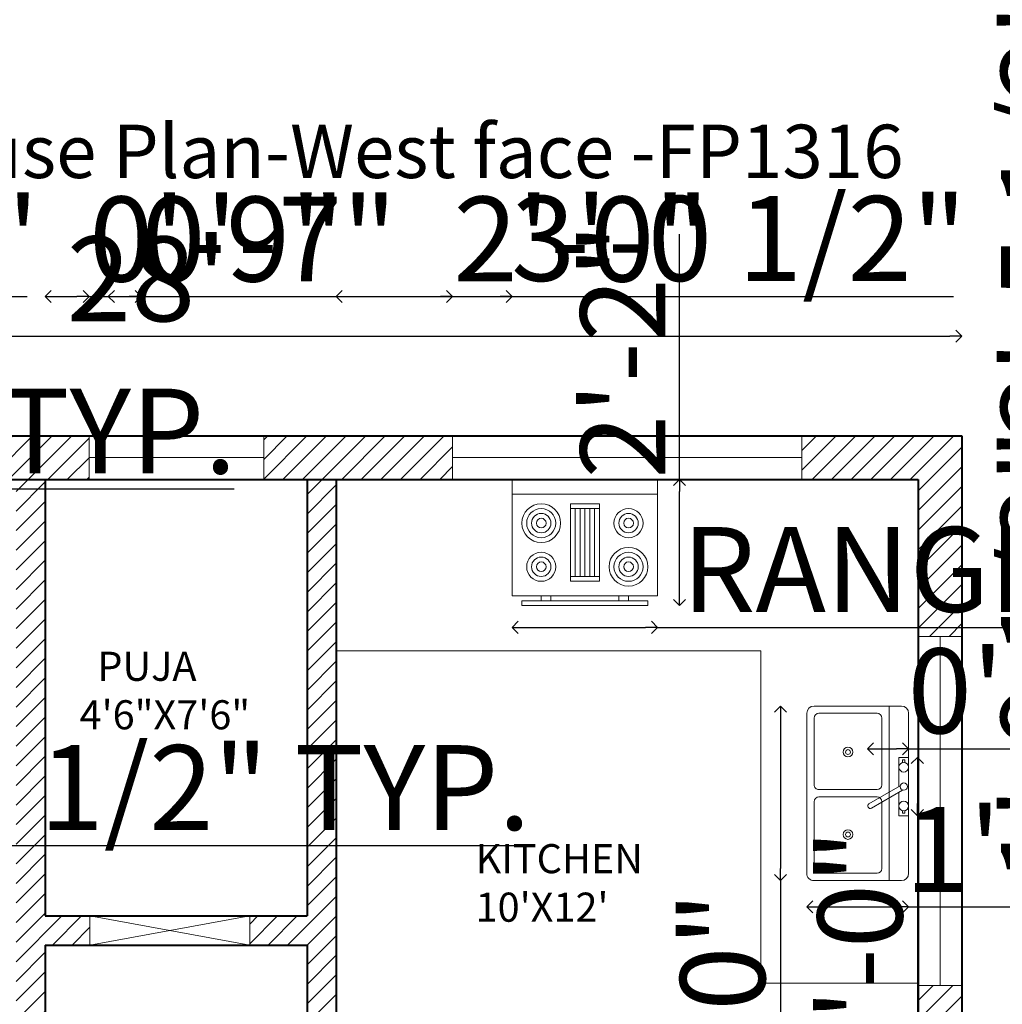
# Model space of a CAD drawing. Units: inches. Extents: x 597 to 1323, y 1833 to 2686.
# Tile 7 of 10: x 914 to 1116, y 2306 to 2509. Entities that reach past the tile are written whole.
import ezdxf

# ---------------------------------------------------------------- set-up
doc = ezdxf.new("R2010")
doc.units = ezdxf.units.IN
for name, color, linetype, lineweight in [('A-ANNO-DIMS', 2, 'Continuous', 18), ('A-ANNO-TEXT', 7, 'Continuous', 18), ('A-AREA-IDEN', 7, 'Continuous', 18), ('A-DOOR', 5, 'Continuous', 20), ('A-FLOR-FIXT', 4, 'Continuous', 18), ('A-GLAZ', 2, 'Continuous', 18), ('A-WALL', 7, 'Continuous', 40), ('A-WALL-PATT', 8, 'Continuous', 13), ('KITCHEN', 4, 'Continuous', 18)]:
    doc.layers.add(name, color=color, linetype=linetype, lineweight=lineweight)
doc.styles.get("Standard").update_dxf_attribs({"font": 'arial.ttf'})
doc.dimstyles.new('ISO-25', dxfattribs={"dimtxt": 17.5, "dimasz": 2.5, "dimexe": 0, "dimexo": 0, "dimtad": 1, "dimdec": 1, "dimlunit": 3, "dimtxsty": 'Standard', "dimblk": 'OPEN90', "dimcen": 2.5, "dimadec": 0, "dimazin": 0, "dimtfac": 1, "dimtdec": 1, "dimtmove": 0, "dimatfit": 3, "dimfxl": 0, "dimfxlon": 1, "dimarcsym": 0})

# ---------------------------------------------------------------- blocks, each defined once
blk = doc.blocks.new('Sink-double - 36 in top')
for p, q in [((-18, -4), (18, -4)), ((-0.75, -18.5), (-0.75, -6.5)), ((0.75, -6.5), (0.75, -18.5))]:
    blk.add_line(p, q)
for points in [[(-16.5, 0), (16.5, 0)], [(-18, -19.5), (-18, -1.5)], [(18, -1.5), (18, -19.5)], [(-15.5, -5.5), (-1.75, -5.5)], [(1.75, -5.5), (15.5, -5.5)], [(-16.5, -18.5), (-16.5, -6.5)], [(16.5, -6.5), (16.5, -18.5)], [(-1.75, -19.5), (-15.5, -19.5)], [(15.5, -19.5), (1.75, -19.5)], [(16.5, -21), (-16.5, -21)]]:
    blk.add_lwpolyline(points)
for centre, radius in [((-8.5, -12.5), 1), ((-8.5, -12.5), 0.5), ((8.5, -12.5), 1), ((8.5, -12.5), 0.5)]:
    blk.add_circle(centre, radius)
for centre, radius, start, end in [((-16.5, -1.5), 1.5, 90, 180), ((16.5, -1.5), 1.5, 0, 90), ((-15.5, -6.5), 1, 90, 180), ((-1.75, -6.5), 1, 0, 90), ((1.75, -6.5), 1, 90, 180), ((15.5, -6.5), 1, 0, 90), ((-16.5, -19.5), 1.5, 180, 270), ((-15.5, -18.5), 1, 180, 270), ((-1.75, -18.5), 1, 270, 0), ((1.75, -18.5), 1, 180, 270), ((15.5, -18.5), 1, 270, 0), ((16.5, -19.5), 1.5, 270, 0)]:
    blk.add_arc(centre, radius, start, end)
blk = doc.blocks.new('Faucet - kit sink top')
for p, q in [((-5.5, -0.75), (-5.5, -1.25)), ((-4.94278, -0.75), (-5.5, -0.75)), ((-5.5, -1.25), (-4.94278, -1.25)), ((-0.14775, -1.7441), (3.56698, -8.1782)), ((4.43301, -7.6782), (0.71828, -1.2441)), ((4.94278, -0.75), (5.5, -0.75)), ((5.5, -1.25), (4.94278, -1.25)), ((5.5, -0.75), (5.5, -1.25))]:
    blk.add_line(p, q)
blk.add_lwpolyline([(-0.00587, -2), (-6, -2), (-6, 0), (6, 0), (6, -2), (1.15195, -2)])
for centre, radius in [((-4, -1), 1), ((4, -1), 1), ((0, -1), 0.75)]:
    blk.add_circle(centre, radius)
blk.add_arc((4, -7.9282), 0.5, 210, 30)
blk = doc.blocks.new('Range-Oven - 30 in top')
for p, q in [((0, -3), (30, -3)), ((12, -6), (18, -6)), ((13, -20), (13, -6)), ((14, -6), (14, -20)), ((15, -20), (15, -6)), ((16, -6), (16, -20)), ((17, -20), (17, -6)), ((18, -20), (12, -20)), ((6, -24), (6, -25)), ((8, -25), (8, -24)), ((22, -25), (22, -24)), ((24, -24), (24, -25))]:
    blk.add_line(p, q)
for points in [[(0, -24), (0, 0), (30, 0), (30, -24)], [(12, -21), (12, -5), (18, -5), (18, -21)], [(2, -26), (2, -25), (28, -25), (28, -26)]]:
    blk.add_lwpolyline(points, close=True)
for centre, radius in [((6, -9), 4), ((6, -9), 3), ((24, -9), 3), ((6, -9), 2), ((6, -9), 1), ((24, -9), 2), ((24, -9), 1), ((24, -18), 4), ((6, -18), 3), ((6, -18), 2), ((24, -18), 3), ((24, -18), 2), ((6, -18), 1), ((24, -18), 1)]:
    blk.add_circle(centre, radius)
blk = doc.blocks.new('_Open90')
at = {"color": 0, "linetype": 'ByBlock', "lineweight": -2}
for p, q in [((0, 0), (-1, 0)), ((-0.5, 0.5), (0, 0)), ((0, 0), (-0.5, -0.5))]:
    blk.add_line(p, q, dxfattribs=at)
blk = doc.blocks.new('*D21')
at = {"layer": 'A-ANNO-DIMS', "color": 0, "lineweight": -2, "transparency": 16777216}
blk.add_line((774.39, 2444.15), (1105.39, 2444.15), dxfattribs=at)
at = {"layer": 'Defpoints', "color": 0, "transparency": 16777216}
for p in [(1107.89, 2444.15), (771.89, 2423.61), (1107.89, 2423.61)]:
    blk.add_point(p, dxfattribs=at)
at = {"layer": 'A-ANNO-DIMS', "color": 0, "lineweight": -2, "transparency": 16777216, "xscale": 2.5, "yscale": 2.5, "zscale": 2.5, "rotation": 180}
blk.add_blockref('_Open90', (771.89, 2444.15), dxfattribs=at)
at = {"layer": 'A-ANNO-DIMS', "color": 0, "lineweight": -2, "transparency": 16777216, "xscale": 2.5, "yscale": 2.5, "zscale": 2.5}
blk.add_blockref('_Open90', (1107.89, 2444.15), dxfattribs=at)
at = {"layer": 'A-ANNO-DIMS', "color": 0, "transparency": 16777216, "insert": (939.89, 2453.71), "char_height": 17.5, "attachment_point": 5}
blk.add_mtext("28'", dxfattribs=at)
blk = doc.blocks.new('*D22')
at = {"layer": 'A-ANNO-DIMS', "color": 0, "lineweight": -2, "transparency": 16777216}
blk.add_line((1136.67, 2421.11), (1136.67, 1946.11), dxfattribs=at)
at = {"layer": 'Defpoints', "color": 0, "transparency": 16777216}
for p in [(1107.89, 2423.61), (1107.89, 1943.61), (1136.67, 1943.61)]:
    blk.add_point(p, dxfattribs=at)
at = {"layer": 'A-ANNO-DIMS', "color": 0, "lineweight": -2, "transparency": 16777216, "xscale": 2.5, "yscale": 2.5, "zscale": 2.5}
for p, rotation in [((1136.67, 2423.61), 90), ((1136.67, 1943.61), 270)]:
    blk.add_blockref('_Open90', p, dxfattribs=dict(at, rotation=rotation))
at = {"layer": 'A-ANNO-DIMS', "color": 0, "transparency": 16777216, "insert": (1127.11, 2183.61), "char_height": 17.5, "attachment_point": 5, "rotation": 90}
blk.add_mtext("40'", dxfattribs=at)
blk = doc.blocks.new('WINDOW-72IN')
for p, q in [((0, 0), (0, 9)), ((72, 0), (72, 9)), ((0, 4.5), (72, 4.5))]:
    blk.add_line(p, q)
blk = doc.blocks.new('WINDOW-36IN')
for p, q in [((0, 0), (0, 9)), ((36, 0), (36, 9)), ((0, 4.5), (36, 4.5))]:
    blk.add_line(p, q)
blk = doc.blocks.new('*D31')
at = {"layer": 'A-ANNO-DIMS', "color": 0, "lineweight": -2, "transparency": 16777216}
for p, q in [((878.8, 2220.09), (878.8, 2504.86)), ((878.8, 2197.8), (878.8, 2217.59))]:
    blk.add_line(p, q, dxfattribs=at)
at = {"layer": 'Defpoints', "color": 0, "transparency": 16777216}
for p in [(875.08, 2220.09), (878.8, 2220.09), (875.08, 2195.3)]:
    blk.add_point(p, dxfattribs=at)
at = {"layer": 'A-ANNO-DIMS', "color": 0, "lineweight": -2, "transparency": 16777216, "xscale": 2.5, "yscale": 2.5, "zscale": 2.5}
for p, rotation in [((878.8, 2220.09), 90), ((878.8, 2195.3), 270)]:
    blk.add_blockref('_Open90', p, dxfattribs=dict(at, rotation=rotation))
at = {"layer": 'A-ANNO-DIMS', "color": 0, "transparency": 16777216, "insert": (869.12, 2363.73), "char_height": 17.5, "attachment_point": 5, "rotation": 90}
blk.add_mtext('DINING CHAIR 2\'-1" TYP.', dxfattribs=at)
blk = doc.blocks.new('*D34')
at = {"layer": 'A-ANNO-DIMS', "color": 0, "lineweight": -2, "transparency": 16777216}
for p, q in [((795.3, 2412.65), (805.8, 2412.65)), ((808.3, 2412.65), (957.85, 2412.65))]:
    blk.add_line(p, q, dxfattribs=at)
at = {"layer": 'Defpoints', "color": 0, "transparency": 16777216}
for p in [(808.3, 2412.65), (792.8, 2410.26), (808.3, 2410.26)]:
    blk.add_point(p, dxfattribs=at)
at = {"layer": 'A-ANNO-DIMS', "color": 0, "lineweight": -2, "transparency": 16777216, "xscale": 2.5, "yscale": 2.5, "zscale": 2.5, "rotation": 180}
blk.add_blockref('_Open90', (792.8, 2412.65), dxfattribs=at)
at = {"layer": 'A-ANNO-DIMS', "color": 0, "lineweight": -2, "transparency": 16777216, "xscale": 2.5, "yscale": 2.5, "zscale": 2.5}
blk.add_blockref('_Open90', (808.3, 2412.65), dxfattribs=at)
at = {"layer": 'A-ANNO-DIMS', "color": 0, "transparency": 16777216, "insert": (884.33, 2422.33), "char_height": 17.5, "attachment_point": 5}
blk.add_mtext('1\'-3 1/2" TYP.', dxfattribs=at)
blk = doc.blocks.new('*D37')
at = {"layer": 'A-ANNO-DIMS', "color": 0, "lineweight": -2, "transparency": 16777216}
for p, q in [((975.39, 2271.58), (999.89, 2271.58)), ((1002.39, 2271.58), (1323.28, 2271.58))]:
    blk.add_line(p, q, dxfattribs=at)
at = {"layer": 'Defpoints', "color": 0, "transparency": 16777216}
for p in [(972.89, 2276), (1002.39, 2276), (1002.39, 2271.58)]:
    blk.add_point(p, dxfattribs=at)
at = {"layer": 'A-ANNO-DIMS', "color": 0, "lineweight": -2, "transparency": 16777216, "xscale": 2.5, "yscale": 2.5, "zscale": 2.5, "rotation": 180}
blk.add_blockref('_Open90', (972.89, 2271.58), dxfattribs=at)
at = {"layer": 'A-ANNO-DIMS', "color": 0, "lineweight": -2, "transparency": 16777216, "xscale": 2.5, "yscale": 2.5, "zscale": 2.5}
blk.add_blockref('_Open90', (1002.39, 2271.58), dxfattribs=at)
at = {"layer": 'A-ANNO-DIMS', "color": 0, "transparency": 16777216, "insert": (1164.08, 2281.25), "char_height": 17.5, "attachment_point": 5}
blk.add_mtext('SWING DOOR 2\'-5 1/2" TYP.', dxfattribs=at)
blk = doc.blocks.new('*D42')
at = {"layer": 'A-ANNO-DIMS', "color": 0, "lineweight": -2, "transparency": 16777216}
for p, q in [((810.8, 2339.13), (852.19, 2339.13)), ((854.69, 2339.13), (1019.47, 2339.13))]:
    blk.add_line(p, q, dxfattribs=at)
at = {"layer": 'Defpoints', "color": 0, "transparency": 16777216}
for p in [(808.3, 2348.41), (854.69, 2348.41), (854.69, 2339.13)]:
    blk.add_point(p, dxfattribs=at)
at = {"layer": 'A-ANNO-DIMS', "color": 0, "lineweight": -2, "transparency": 16777216, "xscale": 2.5, "yscale": 2.5, "zscale": 2.5, "rotation": 180}
blk.add_blockref('_Open90', (808.3, 2339.13), dxfattribs=at)
at = {"layer": 'A-ANNO-DIMS', "color": 0, "lineweight": -2, "transparency": 16777216, "xscale": 2.5, "yscale": 2.5, "zscale": 2.5}
blk.add_blockref('_Open90', (854.69, 2339.13), dxfattribs=at)
at = {"layer": 'A-ANNO-DIMS', "color": 0, "transparency": 16777216, "insert": (938.33, 2348.81), "char_height": 17.5, "attachment_point": 5}
blk.add_mtext('3\'-10 1/2" TYP.', dxfattribs=at)
blk = doc.blocks.new('*D47')
at = {"layer": 'A-ANNO-DIMS', "color": 0, "lineweight": -2, "transparency": 16777216}
for p, q in [((1070.51, 2365.4), (1070.51, 2334.4)), ((1070.51, 2331.9), (1070.51, 2217.86))]:
    blk.add_line(p, q, dxfattribs=at)
at = {"layer": 'Defpoints', "color": 0, "transparency": 16777216}
for p in [(1075.91, 2367.9), (1070.51, 2331.9), (1075.91, 2331.9)]:
    blk.add_point(p, dxfattribs=at)
at = {"layer": 'A-ANNO-DIMS', "color": 0, "lineweight": -2, "transparency": 16777216, "xscale": 2.5, "yscale": 2.5, "zscale": 2.5}
for p, rotation in [((1070.51, 2367.9), 90), ((1070.51, 2331.9), 270)]:
    blk.add_blockref('_Open90', p, dxfattribs=dict(at, rotation=rotation))
at = {"layer": 'A-ANNO-DIMS', "color": 0, "transparency": 16777216, "insert": (1060.83, 2273.63), "char_height": 17.5, "attachment_point": 5, "rotation": 90}
blk.add_mtext('SINK 3\'-0"', dxfattribs=at)
blk = doc.blocks.new('*D48')
at = {"layer": 'A-ANNO-DIMS', "color": 0, "lineweight": -2, "transparency": 16777216}
for p, q in [((1078.41, 2326.5), (1094.41, 2326.5)), ((1096.91, 2326.5), (1145.53, 2326.5))]:
    blk.add_line(p, q, dxfattribs=at)
at = {"layer": 'Defpoints', "color": 0, "transparency": 16777216}
for p in [(1075.91, 2331.9), (1096.91, 2331.9), (1096.91, 2326.5)]:
    blk.add_point(p, dxfattribs=at)
at = {"layer": 'A-ANNO-DIMS', "color": 0, "lineweight": -2, "transparency": 16777216, "xscale": 2.5, "yscale": 2.5, "zscale": 2.5, "rotation": 180}
blk.add_blockref('_Open90', (1075.91, 2326.5), dxfattribs=at)
at = {"layer": 'A-ANNO-DIMS', "color": 0, "lineweight": -2, "transparency": 16777216, "xscale": 2.5, "yscale": 2.5, "zscale": 2.5}
blk.add_blockref('_Open90', (1096.91, 2326.5), dxfattribs=at)
at = {"layer": 'A-ANNO-DIMS', "color": 0, "transparency": 16777216, "insert": (1122.47, 2336.06), "char_height": 17.5, "attachment_point": 5}
blk.add_mtext('1\'-9"', dxfattribs=at)
blk = doc.blocks.new('*D49')
at = {"layer": 'A-ANNO-DIMS', "color": 0, "lineweight": -2, "transparency": 16777216}
for p, q in [((1098.71, 2354.78), (1098.71, 2347.78)), ((1098.71, 2345.28), (1098.71, 2240.23))]:
    blk.add_line(p, q, dxfattribs=at)
at = {"layer": 'Defpoints', "color": 0, "transparency": 16777216}
for p in [(1096.91, 2357.28), (1096.91, 2345.28), (1098.71, 2345.28)]:
    blk.add_point(p, dxfattribs=at)
at = {"layer": 'A-ANNO-DIMS', "color": 0, "lineweight": -2, "transparency": 16777216, "xscale": 2.5, "yscale": 2.5, "zscale": 2.5}
for p, rotation in [((1098.71, 2357.28), 90), ((1098.71, 2345.28), 270)]:
    blk.add_blockref('_Open90', p, dxfattribs=dict(at, rotation=rotation))
at = {"layer": 'A-ANNO-DIMS', "color": 0, "transparency": 16777216, "insert": (1089.15, 2291.5), "char_height": 17.5, "attachment_point": 5, "rotation": 90}
blk.add_mtext('TAP 1\'-0"', dxfattribs=at)
blk = doc.blocks.new('*D50')
at = {"layer": 'A-ANNO-DIMS', "color": 0, "lineweight": -2, "transparency": 16777216}
for p, q in [((1090.91, 2359.08), (1094.41, 2359.08)), ((1096.91, 2359.08), (1187.96, 2359.08))]:
    blk.add_line(p, q, dxfattribs=at)
at = {"layer": 'Defpoints', "color": 0, "transparency": 16777216}
for p in [(1088.41, 2357.28), (1096.91, 2359.08), (1096.91, 2357.28)]:
    blk.add_point(p, dxfattribs=at)
at = {"layer": 'A-ANNO-DIMS', "color": 0, "lineweight": -2, "transparency": 16777216, "xscale": 2.5, "yscale": 2.5, "zscale": 2.5, "rotation": 180}
blk.add_blockref('_Open90', (1088.41, 2359.08), dxfattribs=at)
at = {"layer": 'A-ANNO-DIMS', "color": 0, "lineweight": -2, "transparency": 16777216, "xscale": 2.5, "yscale": 2.5, "zscale": 2.5}
blk.add_blockref('_Open90', (1096.91, 2359.08), dxfattribs=at)
at = {"layer": 'A-ANNO-DIMS', "color": 0, "transparency": 16777216, "insert": (1143.68, 2368.75), "char_height": 17.5, "attachment_point": 5}
blk.add_mtext('0\'-8 1/2"', dxfattribs=at)
blk = doc.blocks.new('*D53')
at = {"layer": 'A-ANNO-DIMS', "color": 0, "lineweight": -2, "transparency": 16777216}
for p, q in [((1017.66, 2384.11), (1042.66, 2384.11)), ((1045.16, 2384.11), (1188.25, 2384.11))]:
    blk.add_line(p, q, dxfattribs=at)
at = {"layer": 'Defpoints', "color": 0, "transparency": 16777216}
for p in [(1015.16, 2388.61), (1045.16, 2388.61), (1045.16, 2384.11)]:
    blk.add_point(p, dxfattribs=at)
at = {"layer": 'A-ANNO-DIMS', "color": 0, "lineweight": -2, "transparency": 16777216, "xscale": 2.5, "yscale": 2.5, "zscale": 2.5, "rotation": 180}
blk.add_blockref('_Open90', (1015.16, 2384.11), dxfattribs=at)
at = {"layer": 'A-ANNO-DIMS', "color": 0, "lineweight": -2, "transparency": 16777216, "xscale": 2.5, "yscale": 2.5, "zscale": 2.5}
blk.add_blockref('_Open90', (1045.16, 2384.11), dxfattribs=at)
at = {"layer": 'A-ANNO-DIMS', "color": 0, "transparency": 16777216, "insert": (1117.95, 2393.78), "char_height": 17.5, "attachment_point": 5}
blk.add_mtext('RANGE 2\'-6"', dxfattribs=at)
blk = doc.blocks.new('*D54')
at = {"layer": 'A-ANNO-DIMS', "color": 0, "lineweight": -2, "transparency": 16777216}
for p, q in [((1049.66, 2414.61), (1049.66, 2465.18)), ((1049.66, 2391.11), (1049.66, 2412.11))]:
    blk.add_line(p, q, dxfattribs=at)
at = {"layer": 'Defpoints', "color": 0, "transparency": 16777216}
for p in [(1045.16, 2414.61), (1049.66, 2414.61), (1045.16, 2388.61)]:
    blk.add_point(p, dxfattribs=at)
at = {"layer": 'A-ANNO-DIMS', "color": 0, "lineweight": -2, "transparency": 16777216, "xscale": 2.5, "yscale": 2.5, "zscale": 2.5}
for p, rotation in [((1049.66, 2414.61), 90), ((1049.66, 2388.61), 270)]:
    blk.add_blockref('_Open90', p, dxfattribs=dict(at, rotation=rotation))
at = {"layer": 'A-ANNO-DIMS', "color": 0, "transparency": 16777216, "insert": (1040.24, 2441.14), "char_height": 17.5, "attachment_point": 5, "rotation": 90}
blk.add_mtext('2\'-2"', dxfattribs=at)
blk = doc.blocks.new('*D55')
at = {"layer": 'A-ANNO-DIMS', "color": 0, "lineweight": -2, "transparency": 16777216}
for p, q in [((825.39, 2452.36), (862.39, 2452.36)), ((864.89, 2452.36), (915.14, 2452.36))]:
    blk.add_line(p, q, dxfattribs=at)
at = {"layer": 'Defpoints', "color": 0, "transparency": 16777216}
for p in [(864.89, 2452.36), (822.89, 2075.33), (864.89, 2075.33)]:
    blk.add_point(p, dxfattribs=at)
at = {"layer": 'A-ANNO-DIMS', "color": 0, "lineweight": -2, "transparency": 16777216, "xscale": 2.5, "yscale": 2.5, "zscale": 2.5, "rotation": 180}
blk.add_blockref('_Open90', (822.89, 2452.36), dxfattribs=at)
at = {"layer": 'A-ANNO-DIMS', "color": 0, "lineweight": -2, "transparency": 16777216, "xscale": 2.5, "yscale": 2.5, "zscale": 2.5}
blk.add_blockref('_Open90', (864.89, 2452.36), dxfattribs=at)
at = {"layer": 'A-ANNO-DIMS', "color": 0, "transparency": 16777216, "insert": (891.27, 2461.93), "char_height": 17.5, "attachment_point": 5}
blk.add_mtext('3\'-6"', dxfattribs=at)
blk = doc.blocks.new('*D62')
at = {"layer": 'A-ANNO-DIMS', "color": 0, "lineweight": -2, "transparency": 16777216}
for p, q in [((981.39, 2452.36), (1000.39, 2452.36)), ((1002.89, 2452.36), (1053.45, 2452.36))]:
    blk.add_line(p, q, dxfattribs=at)
at = {"layer": 'Defpoints', "color": 0, "transparency": 16777216}
for p in [(1002.89, 2452.36), (978.89, 2414.61), (1002.89, 2414.61)]:
    blk.add_point(p, dxfattribs=at)
at = {"layer": 'A-ANNO-DIMS', "color": 0, "lineweight": -2, "transparency": 16777216, "xscale": 2.5, "yscale": 2.5, "zscale": 2.5, "rotation": 180}
blk.add_blockref('_Open90', (978.89, 2452.36), dxfattribs=at)
at = {"layer": 'A-ANNO-DIMS', "color": 0, "lineweight": -2, "transparency": 16777216, "xscale": 2.5, "yscale": 2.5, "zscale": 2.5}
blk.add_blockref('_Open90', (1002.89, 2452.36), dxfattribs=at)
at = {"layer": 'A-ANNO-DIMS', "color": 0, "transparency": 16777216, "insert": (1029.42, 2461.92), "char_height": 17.5, "attachment_point": 5}
blk.add_mtext('2\'-0"', dxfattribs=at)
blk = doc.blocks.new('*D63')
at = {"layer": 'A-ANNO-DIMS', "color": 0, "lineweight": -2, "transparency": 16777216}
for p, q in [((921.39, 2452.36), (925.43, 2452.36)), ((927.93, 2452.36), (978.2, 2452.36))]:
    blk.add_line(p, q, dxfattribs=at)
at = {"layer": 'Defpoints', "color": 0, "transparency": 16777216}
for p in [(927.93, 2452.36), (918.89, 2414.61), (927.93, 2414.61)]:
    blk.add_point(p, dxfattribs=at)
at = {"layer": 'A-ANNO-DIMS', "color": 0, "lineweight": -2, "transparency": 16777216, "xscale": 2.5, "yscale": 2.5, "zscale": 2.5, "rotation": 180}
blk.add_blockref('_Open90', (918.89, 2452.36), dxfattribs=at)
at = {"layer": 'A-ANNO-DIMS', "color": 0, "lineweight": -2, "transparency": 16777216, "xscale": 2.5, "yscale": 2.5, "zscale": 2.5}
blk.add_blockref('_Open90', (927.93, 2452.36), dxfattribs=at)
at = {"layer": 'A-ANNO-DIMS', "color": 0, "transparency": 16777216, "insert": (954.31, 2461.92), "char_height": 17.5, "attachment_point": 5}
blk.add_mtext('0\'-9"', dxfattribs=at)
blk = doc.blocks.new('*D64')
at = {"layer": 'A-ANNO-DIMS', "color": 0, "lineweight": -2, "transparency": 16777216}
for p, q in [((1136.64, 2423.61), (1136.64, 2514.65)), ((1136.64, 2384.76), (1136.64, 2421.11))]:
    blk.add_line(p, q, dxfattribs=at)
at = {"layer": 'Defpoints', "color": 0, "transparency": 16777216}
for p in [(1107.89, 2423.61), (1136.64, 2423.61), (1107.89, 2382.26)]:
    blk.add_point(p, dxfattribs=at)
at = {"layer": 'A-ANNO-DIMS', "color": 0, "lineweight": -2, "transparency": 16777216, "xscale": 2.5, "yscale": 2.5, "zscale": 2.5}
for p, rotation in [((1136.64, 2423.61), 90), ((1136.64, 2382.26), 270)]:
    blk.add_blockref('_Open90', p, dxfattribs=dict(at, rotation=rotation))
at = {"layer": 'A-ANNO-DIMS', "color": 0, "transparency": 16777216, "insert": (1126.96, 2470.38), "char_height": 17.5, "attachment_point": 5, "rotation": 90}
blk.add_mtext('3\'-5 1/2"', dxfattribs=at)
blk = doc.blocks.new('*D69')
at = {"layer": 'A-ANNO-DIMS', "color": 0, "lineweight": -2, "transparency": 16777216}
for p, q in [((743.14, 2412.11), (743.14, 2381.8)), ((743.14, 2379.3), (743.14, 2274.36))]:
    blk.add_line(p, q, dxfattribs=at)
at = {"layer": 'Defpoints', "color": 0, "transparency": 16777216}
for p in [(978.89, 2414.61), (743.14, 2379.3), (978.89, 2379.3)]:
    blk.add_point(p, dxfattribs=at)
at = {"layer": 'A-ANNO-DIMS', "color": 0, "lineweight": -2, "transparency": 16777216, "xscale": 2.5, "yscale": 2.5, "zscale": 2.5}
for p, rotation in [((743.14, 2414.61), 90), ((743.14, 2379.3), 270)]:
    blk.add_blockref('_Open90', p, dxfattribs=dict(at, rotation=rotation))
at = {"layer": 'A-ANNO-DIMS', "color": 0, "transparency": 16777216, "insert": (733.46, 2325.58), "char_height": 17.5, "attachment_point": 5, "rotation": 90}
blk.add_mtext('2\'-11 1/2"', dxfattribs=at)
blk = doc.blocks.new('*D70')
at = {"layer": 'A-ANNO-DIMS', "color": 0, "lineweight": -2, "transparency": 16777216}
for p, q in [((1066.43, 1912.53), (975.08, 1912.53)), ((1096.39, 1912.53), (1068.93, 1912.53))]:
    blk.add_line(p, q, dxfattribs=at)
at = {"layer": 'Defpoints', "color": 0, "transparency": 16777216}
for p in [(1066.43, 2310.73), (1098.89, 2310.73), (1066.43, 1912.53)]:
    blk.add_point(p, dxfattribs=at)
at = {"layer": 'A-ANNO-DIMS', "color": 0, "lineweight": -2, "transparency": 16777216, "xscale": 2.5, "yscale": 2.5, "zscale": 2.5, "rotation": 180}
blk.add_blockref('_Open90', (1066.43, 1912.53), dxfattribs=at)
at = {"layer": 'A-ANNO-DIMS', "color": 0, "lineweight": -2, "transparency": 16777216, "xscale": 2.5, "yscale": 2.5, "zscale": 2.5}
blk.add_blockref('_Open90', (1098.89, 1912.53), dxfattribs=at)
at = {"layer": 'A-ANNO-DIMS', "color": 0, "transparency": 16777216, "insert": (1019.5, 1922.21), "char_height": 17.5, "attachment_point": 5}
blk.add_mtext('2\'-8 1/2"', dxfattribs=at)
blk = doc.blocks.new('*D71')
at = {"layer": 'A-ANNO-DIMS', "color": 0, "lineweight": -2, "transparency": 16777216}
for p, q in [((743.14, 2379.3), (743.14, 2470.35)), ((743.14, 2313.23), (743.14, 2376.8))]:
    blk.add_line(p, q, dxfattribs=at)
at = {"layer": 'Defpoints', "color": 0, "transparency": 16777216}
for p in [(743.14, 2379.3), (1066.43, 2379.3), (1066.43, 2310.73)]:
    blk.add_point(p, dxfattribs=at)
at = {"layer": 'A-ANNO-DIMS', "color": 0, "lineweight": -2, "transparency": 16777216, "xscale": 2.5, "yscale": 2.5, "zscale": 2.5}
for p, rotation in [((743.14, 2379.3), 90), ((743.14, 2310.73), 270)]:
    blk.add_blockref('_Open90', p, dxfattribs=dict(at, rotation=rotation))
at = {"layer": 'A-ANNO-DIMS', "color": 0, "transparency": 16777216, "insert": (733.46, 2426.07), "char_height": 17.5, "attachment_point": 5, "rotation": 90}
blk.add_mtext('5\'-8 1/2"', dxfattribs=at)
blk = doc.blocks.new('*D72')
at = {"layer": 'A-ANNO-DIMS', "color": 0, "lineweight": -2, "transparency": 16777216}
for p, q in [((981.39, 2452.36), (1012.66, 2452.36)), ((1015.16, 2452.36), (1106.19, 2452.36))]:
    blk.add_line(p, q, dxfattribs=at)
at = {"layer": 'Defpoints', "color": 0, "transparency": 16777216}
for p in [(1015.16, 2452.36), (978.89, 2414.61), (1015.16, 2414.61)]:
    blk.add_point(p, dxfattribs=at)
at = {"layer": 'A-ANNO-DIMS', "color": 0, "lineweight": -2, "transparency": 16777216, "xscale": 2.5, "yscale": 2.5, "zscale": 2.5, "rotation": 180}
blk.add_blockref('_Open90', (978.89, 2452.36), dxfattribs=at)
at = {"layer": 'A-ANNO-DIMS', "color": 0, "lineweight": -2, "transparency": 16777216, "xscale": 2.5, "yscale": 2.5, "zscale": 2.5}
blk.add_blockref('_Open90', (1015.16, 2452.36), dxfattribs=at)
at = {"layer": 'A-ANNO-DIMS', "color": 0, "transparency": 16777216, "insert": (1061.92, 2462.04), "char_height": 17.5, "attachment_point": 5}
blk.add_mtext('3\'-0 1/2"', dxfattribs=at)
blk = doc.blocks.new('*D73')
at = {"layer": 'A-ANNO-DIMS', "color": 0, "lineweight": -2, "transparency": 16777216}
for p, q in [((1136.64, 2332.34), (1136.64, 2421.74)), ((1136.64, 2313.23), (1136.64, 2329.84))]:
    blk.add_line(p, q, dxfattribs=at)
at = {"layer": 'Defpoints', "color": 0, "transparency": 16777216}
for p in [(1096.47, 2332.34), (1136.64, 2332.34), (1098.89, 2310.73)]:
    blk.add_point(p, dxfattribs=at)
at = {"layer": 'A-ANNO-DIMS', "color": 0, "lineweight": -2, "transparency": 16777216, "xscale": 2.5, "yscale": 2.5, "zscale": 2.5}
for p, rotation in [((1136.64, 2332.34), 90), ((1136.64, 2310.73), 270)]:
    blk.add_blockref('_Open90', p, dxfattribs=dict(at, rotation=rotation))
at = {"layer": 'A-ANNO-DIMS', "color": 0, "transparency": 16777216, "insert": (1126.96, 2378.29), "char_height": 17.5, "attachment_point": 5, "rotation": 90}
blk.add_mtext('1\'-9 1/2"', dxfattribs=at)
blk = doc.blocks.new('*D80')
at = {"layer": 'A-ANNO-DIMS', "color": 0, "lineweight": -2, "transparency": 16777216}
for p, q in [((743.14, 2278.5), (743.14, 2369.55)), ((743.14, 2270.61), (743.14, 2276)), ((743.14, 2268.11), (743.14, 2265.61))]:
    blk.add_line(p, q, dxfattribs=at)
at = {"layer": 'Defpoints', "color": 0, "transparency": 16777216}
for p in [(743.14, 2276), (978.89, 2276), (978.89, 2270.61)]:
    blk.add_point(p, dxfattribs=at)
at = {"layer": 'A-ANNO-DIMS', "color": 0, "lineweight": -2, "transparency": 16777216, "xscale": 2.5, "yscale": 2.5, "zscale": 2.5}
for p, rotation in [((743.14, 2276), 270), ((743.14, 2270.61), 90)]:
    blk.add_blockref('_Open90', p, dxfattribs=dict(at, rotation=rotation))
at = {"layer": 'A-ANNO-DIMS', "color": 0, "transparency": 16777216, "insert": (733.46, 2325.27), "char_height": 17.5, "attachment_point": 5, "rotation": 90}
blk.add_mtext('0\'-5 1/2"', dxfattribs=at)
blk = doc.blocks.new('*D82')
at = {"layer": 'A-ANNO-DIMS', "color": 0, "lineweight": -2, "transparency": 16777216}
for p, q in [((934.39, 2452.36), (936.18, 2452.36)), ((938.68, 2452.36), (988.95, 2452.36))]:
    blk.add_line(p, q, dxfattribs=at)
at = {"layer": 'Defpoints', "color": 0, "transparency": 16777216}
for p in [(938.68, 2452.36), (931.89, 2138.61), (938.68, 2138.61)]:
    blk.add_point(p, dxfattribs=at)
at = {"layer": 'A-ANNO-DIMS', "color": 0, "lineweight": -2, "transparency": 16777216, "xscale": 2.5, "yscale": 2.5, "zscale": 2.5, "rotation": 180}
blk.add_blockref('_Open90', (931.89, 2452.36), dxfattribs=at)
at = {"layer": 'A-ANNO-DIMS', "color": 0, "lineweight": -2, "transparency": 16777216, "xscale": 2.5, "yscale": 2.5, "zscale": 2.5}
blk.add_blockref('_Open90', (938.68, 2452.36), dxfattribs=at)
at = {"layer": 'A-ANNO-DIMS', "color": 0, "transparency": 16777216, "insert": (965.06, 2461.92), "char_height": 17.5, "attachment_point": 5}
blk.add_mtext('0\'-7"', dxfattribs=at)

msp = doc.modelspace()

# ---------------------------------------------------------------- hatches: boundary and pattern name
at = {"layer": 'A-WALL-PATT'}
h = msp.add_hatch(dxfattribs=at)
h.set_pattern_fill('ANSI31', color=256, scale=0.9)
h.paths.add_polyline_path([(927.93, 2423.61), (771.89, 2423.61), (771.89, 2371.61), (780.89, 2371.61), (780.89, 2414.61), (918.89, 2414.61), (927.93, 2414.61)])
h.paths.add_polyline_path([(1107.89, 2423.61), (1074.89, 2423.61), (1074.89, 2414.61), (1098.89, 2414.61), (1098.89, 2382.26), (1107.89, 2382.26)])
h.paths.add_polyline_path([(1002.89, 2423.61), (963.93, 2423.61), (963.93, 2414.61), (978.89, 2414.61), (1002.89, 2414.61)])
h.paths.add_polyline_path([(918.89, 2414.61), (912.89, 2414.61), (912.89, 2270.61), (906.2, 2270.61), (906.2, 2264.61), (918.89, 2264.61), (918.89, 2318.61), (928.09, 2318.61), (928.09, 2324.61), (918.89, 2324.61)])
h.paths.add_polyline_path([(780.89, 2299.61), (771.89, 2299.61), (771.89, 2245.99), (780.89, 2245.99)])
h.paths.add_polyline_path([(780.89, 2173.99), (771.89, 2173.99), (771.89, 1943.61), (790.26, 1943.61), (790.26, 1952.61), (780.89, 1952.61)])
h.paths.add_polyline_path([(873.89, 1991.61), (887.56, 1991.61), (887.56, 2000.61), (864.89, 2000.61), (864.89, 1952.61), (857.81, 1952.61), (857.81, 1943.61), (873.89, 1943.61)])
h.paths.add_polyline_path([(979.81, 2000.61), (908.62, 2000.61), (908.62, 1991.61), (979.81, 1991.61)])
h.paths.add_polyline_path([(931.89, 2138.61), (938.68, 2138.61), (938.68, 2144.61), (925.89, 2144.61), (925.89, 2000.61), (931.89, 2000.61)])
h.paths.add_polyline_path([(870.89, 2084.61), (874.89, 2084.61), (874.89, 2090.61), (870.89, 2090.61), (870.89, 2144.61), (815.52, 2144.61), (815.52, 2138.61), (864.89, 2138.61), (864.89, 2000.61), (870.89, 2000.61)])
h.paths.add_polyline_path([(925.89, 2090.61), (900.18, 2090.61), (900.18, 2084.61), (925.89, 2084.61)])
h.paths.add_polyline_path([(1107.89, 2051.2), (1098.89, 2051.2), (1098.89, 2000.61), (1047.65, 2000.61), (1047.65, 1991.61), (1107.89, 1991.61)])
h.paths.add_polyline_path([(1107.89, 2181.44), (1098.89, 2181.44), (1098.89, 2109.76), (1107.89, 2109.76)])
h.paths.add_polyline_path([(1098.89, 2144.61), (978.89, 2144.61), (978.89, 2157.94), (972.89, 2157.94), (972.89, 2144.61), (963.97, 2144.61), (963.97, 2138.61), (1098.89, 2138.61)])
h.paths.add_polyline_path([(1107.89, 2310.26), (1098.89, 2310.26), (1098.89, 2227.53), (1107.89, 2227.53)])
h.paths.add_polyline_path([(1098.89, 2270.61), (978.89, 2270.61), (978.89, 2276), (972.89, 2276), (972.89, 2183.23), (978.89, 2183.23), (978.89, 2264.61), (1098.89, 2264.61)])
h.paths.add_polyline_path([(880.92, 2270.61), (780.89, 2270.61), (780.89, 2264.61), (880.92, 2264.61)])
h.paths.add_polyline_path([(978.89, 2414.61), (972.89, 2414.61), (972.89, 2324.61), (961.07, 2324.61), (961.07, 2318.61), (972.89, 2318.61), (972.89, 2301.29), (978.89, 2301.29)])
h.paths.add_polyline_path([(790.26, 2144.61), (780.89, 2144.61), (780.89, 2138.61), (790.26, 2138.61)], flags=17)

# ---------------------------------------------------------------- linework, layer by layer
at = {"layer": 'A-DOOR'}
for p, q in [((928.09, 2324.61), (928.09, 2318.61)), ((961.07, 2318.61), (928.09, 2324.61)), ((928.09, 2318.61), (961.07, 2324.61)), ((961.07, 2324.61), (961.07, 2318.61))]:
    msp.add_line(p, q, dxfattribs=at)
at = {"layer": 'A-WALL'}
for p, q in [((771.89, 2423.61), (1107.89, 2423.61)), ((1107.89, 2423.61), (1107.89, 1943.61)), ((780.89, 2414.61), (918.89, 2414.61)), ((918.89, 2414.61), (918.89, 2324.61)), ((918.89, 2414.61), (978.89, 2414.61)), ((972.89, 2414.61), (972.89, 2324.61)), ((978.89, 2414.61), (978.89, 2301.27)), ((978.89, 2414.61), (1098.89, 2414.61)), ((1098.89, 2414.61), (1098.89, 2000.61)), ((918.89, 2324.61), (972.89, 2324.61)), ((918.89, 2318.61), (972.89, 2318.61)), ((918.89, 2318.61), (918.89, 2264.61)), ((972.89, 2318.61), (972.89, 2144.61))]:
    msp.add_line(p, q, dxfattribs=at)
at = {"layer": 'KITCHEN'}
for p, q in [((978.89, 2379.3), (978.89, 2379.3)), ((978.89, 2379.3), (1066.43, 2379.3)), ((1066.43, 2379.3), (1066.43, 2310.73)), ((1066.43, 2310.73), (1098.89, 2310.73))]:
    msp.add_line(p, q, dxfattribs=at)
msp.add_lwpolyline([(1008.21, 2414.61), (1008.21, 2414.61), (1008.21, 2414.61), (1008.21, 2414.61)], close=True, dxfattribs=at)

# ---------------------------------------------------------------- block references
at = {"layer": 'A-FLOR-FIXT', "rotation": 270}
for name, p in [('Sink-double - 36 in top', (1096.91, 2349.9)), ('Faucet - kit sink top', (1096.91, 2351.28))]:
    msp.add_blockref(name, p, dxfattribs=at)
at = {"layer": 'A-GLAZ'}
for name, p in [('WINDOW-36IN', (927.93, 2414.61)), ('WINDOW-72IN', (1002.89, 2414.61))]:
    msp.add_blockref(name, p, dxfattribs=at)
at = {"layer": 'A-GLAZ', "rotation": 89.9999999999993}
msp.add_blockref('WINDOW-72IN', (1107.89, 2310.26), dxfattribs=at)
at = {"layer": 'KITCHEN'}
msp.add_blockref('Range-Oven - 30 in top', (1015.16, 2414.61), dxfattribs=at)

# ---------------------------------------------------------------- texts
at = {"layer": 'A-ANNO-TEXT', "insert": (769.38, 2487.77), "char_height": 11, "attachment_point": 1}
msp.add_mtext_dynamic_manual_height_columns('28X40(1120sq ft)House Plan-West face -FP1316', width=624.2346, gutter_width=12.5, heights=[0], dxfattribs=at)
at = {"layer": 'A-AREA-IDEN', "char_height": 6, "attachment_point": 1}
for s, width, insert in [('  PUJA\\P4\'6"X7\'6"', 54.7527, (925.97, 2379.09)), ("KITCHEN\\P10'X12'", 39.0037, (1007.62, 2339.42))]:
    msp.add_mtext_dynamic_manual_height_columns(s, width=width, gutter_width=12.5, heights=[0], dxfattribs=dict(at, insert=insert))

# ---------------------------------------------------------------- dimensions: what is measured, and where the dimension line sits
at = {"layer": 'A-ANNO-DIMS'}
for base, p1, p2, override, picture, middle in [((1136.6363, 2423.6106), (1107.8863, 2382.26), (1107.8863, 2423.6106), {"dimdec": 1, "dimlfac": 1, "dimrnd": 0, "dimzin": 1, "dimdsep": 46, "dimlunit": 4, "dimfrac": 2}, '*D64', (1126.9569, 2470.3782)), ((743.14, 2379.3), (1066.43, 2310.73), (1066.43, 2379.3), {"dimdec": 1, "dimlfac": 1, "dimrnd": 0, "dimzin": 1, "dimdsep": 46, "dimlunit": 4, "dimfrac": 2}, '*D71', (733.46, 2426.07)), ((1049.66, 2414.61), (1045.16, 2388.61), (1045.16, 2414.61), {"dimdec": 1, "dimlfac": 1, "dimrnd": 0, "dimzin": 1, "dimdsep": 46, "dimlunit": 4, "dimfrac": 2}, '*D54', (1040.24, 2441.14)), ((1136.64, 2332.34), (1098.89, 2310.73), (1096.47, 2332.34), {"dimdec": 1, "dimlfac": 1, "dimrnd": 0, "dimzin": 1, "dimdsep": 46, "dimlunit": 4, "dimfrac": 2}, '*D73', (1126.96, 2378.29)), ((1136.67, 1943.61), (1107.89, 2423.61), (1107.89, 1943.61), {"dimclrd": 0, "dimclre": 0, "dimclrt": 0}, '*D22', (1127.11, 2183.61)), ((743.14, 2379.3), (978.89, 2414.61), (978.89, 2379.3), {"dimdec": 1, "dimlfac": 1, "dimrnd": 0, "dimzin": 1, "dimdsep": 46, "dimlunit": 4, "dimfrac": 2}, '*D69', (733.46, 2325.58)), ((743.14, 2276), (978.89, 2270.61), (978.89, 2276), {"dimdec": 1, "dimlfac": 1, "dimrnd": 0, "dimzin": 1, "dimdsep": 46, "dimlunit": 4, "dimfrac": 2}, '*D80', (733.46, 2325.27))]:
    dim = msp.add_linear_dim(base=base, p1=p1, p2=p2, angle=90, dimstyle='ISO-25', override=override, dxfattribs=at)
    dim.commit()
    dim.dimension.update_dxf_attribs({"geometry": picture, "text_midpoint": middle})
for base, p1, p2, angle, text, picture, middle in [((878.8, 2220.09), (875.08, 2195.3), (875.08, 2220.09), 90, 'DINING CHAIR <> TYP.', '*D31', (869.12, 2363.73)), ((1070.51, 2331.9), (1075.91, 2367.9), (1075.91, 2331.9), 270, 'SINK <>', '*D47', (1060.83, 2273.63)), ((1098.71, 2345.28), (1096.91, 2357.28), (1096.91, 2345.28), 270, 'TAP <>', '*D49', (1089.15, 2291.5))]:
    dim = msp.add_linear_dim(base=base, p1=p1, p2=p2, angle=angle, text=text, dimstyle='ISO-25', override={"dimdec": 1, "dimlfac": 1, "dimrnd": 0, "dimzin": 1, "dimdsep": 46, "dimlunit": 4, "dimfrac": 2}, dxfattribs=at)
    dim.commit()
    dim.dimension.update_dxf_attribs({"geometry": picture, "text_midpoint": middle})
for base, p1, p2, override, picture, middle in [((1015.16, 2452.36), (978.89, 2414.61), (1015.16, 2414.61), {"dimdec": 1, "dimlfac": 1, "dimrnd": 0, "dimzin": 1, "dimdsep": 46, "dimlunit": 4, "dimfrac": 2}, '*D72', (1061.92, 2462.04)), ((864.89, 2452.36), (822.89, 2075.33), (864.89, 2075.33), {"dimdec": 1, "dimlfac": 1, "dimrnd": 0, "dimzin": 1, "dimdsep": 46, "dimlunit": 4, "dimfrac": 2}, '*D55', (891.27, 2461.93)), ((927.93, 2452.36), (918.89, 2414.61), (927.93, 2414.61), {"dimdec": 1, "dimlfac": 1, "dimrnd": 0, "dimzin": 1, "dimdsep": 46, "dimlunit": 4, "dimfrac": 2}, '*D63', (954.31, 2461.92)), ((938.68, 2452.36), (931.89, 2138.61), (938.68, 2138.61), {"dimdec": 1, "dimlfac": 1, "dimrnd": 0, "dimzin": 1, "dimdsep": 46, "dimlunit": 4, "dimfrac": 2}, '*D82', (965.06, 2461.92)), ((1002.89, 2452.36), (978.89, 2414.61), (1002.89, 2414.61), {"dimdec": 1, "dimlfac": 1, "dimrnd": 0, "dimzin": 1, "dimdsep": 46, "dimlunit": 4, "dimfrac": 2}, '*D62', (1029.42, 2461.92)), ((1107.89, 2444.15), (771.89, 2423.61), (1107.89, 2423.61), {"dimclrd": 0, "dimclre": 0, "dimclrt": 0}, '*D21', (939.89, 2453.71)), ((1096.91, 2359.08), (1088.41, 2357.28), (1096.91, 2357.28), {"dimdec": 1, "dimlfac": 1, "dimrnd": 0, "dimzin": 1, "dimdsep": 46, "dimlunit": 4, "dimfrac": 2}, '*D50', (1143.68, 2368.75)), ((1096.91, 2326.5), (1075.91, 2331.9), (1096.91, 2331.9), {"dimdec": 1, "dimlfac": 1, "dimrnd": 0, "dimzin": 1, "dimdsep": 46, "dimlunit": 4, "dimfrac": 2}, '*D48', (1122.47, 2336.06)), ((1066.43, 1912.53), (1098.89, 2310.73), (1066.43, 2310.73), {"dimdec": 1, "dimlfac": 1, "dimrnd": 0, "dimzin": 1, "dimdsep": 46, "dimlunit": 4, "dimfrac": 2}, '*D70', (1019.5, 1922.21))]:
    dim = msp.add_linear_dim(base=base, p1=p1, p2=p2, dimstyle='ISO-25', override=override, dxfattribs=at)
    dim.commit()
    dim.dimension.update_dxf_attribs({"geometry": picture, "text_midpoint": middle})
for base, p1, p2, text, picture, middle in [((808.3, 2412.65), (792.8, 2410.26), (808.3, 2410.26), '<> TYP.', '*D34', (884.33, 2422.33)), ((1045.16, 2384.11), (1015.16, 2388.61), (1045.16, 2388.61), 'RANGE <>', '*D53', (1117.95, 2393.78)), ((854.69, 2339.13), (808.3, 2348.41), (854.69, 2348.41), '<> TYP.', '*D42', (938.33, 2348.81)), ((1002.39, 2271.58), (972.89, 2276), (1002.39, 2276), 'SWING DOOR <> TYP.', '*D37', (1164.08, 2281.25))]:
    dim = msp.add_linear_dim(base=base, p1=p1, p2=p2, text=text, dimstyle='ISO-25', override={"dimdec": 1, "dimlfac": 1, "dimrnd": 0, "dimzin": 1, "dimdsep": 46, "dimlunit": 4, "dimfrac": 2}, dxfattribs=at)
    dim.commit()
    dim.dimension.update_dxf_attribs({"geometry": picture, "text_midpoint": middle})

doc.saveas('drawing.dxf')
